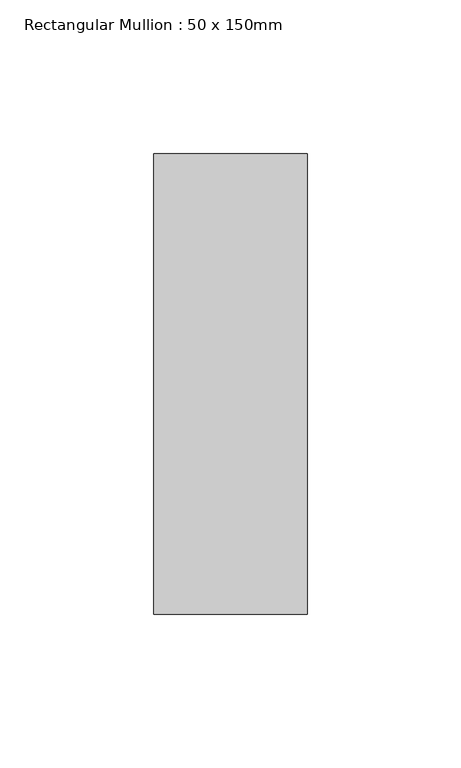
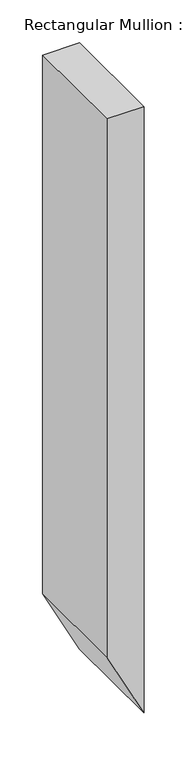
"""IFC4 building model written with IfcOpenShell, lengths in millimetres: member geometry, Rectangular Mullion : 50 x 150mm."""

from ifc_helpers import new_model, si_unit, frame, origin, place, context, project, spatial, polyline, outline, extrude, source, transform, mapped, element, save


def rectangular_mullion_50_x_150mm_a3343b62(model_context):
    return source(origin(), model_context, "Body", "SweptSolid", [
        extrude(outline(polyline([(0.0, 0.0), (0.0, -50.0), (-767.5359884, -50.0), (-863.5850948, 0.0), (0.0, 0.0)])), frame((0.0, -75.0, 0.0), z_axis=(0.0, 1.0, 0.0), x_axis=(0.0, 0.0, 1.0)), (0.0, 0.0, 1.0), 150.0),
    ])


if __name__ == "__main__":
    model = new_model("IFC4")
    model_context = context("Model", 3, world=origin())
    ifc_project = project(units=[si_unit("LENGTHUNIT", "METRE", prefix="MILLI")], contexts=[model_context])
    site = spatial("IfcSite", under=ifc_project)
    building = spatial("IfcBuilding", under=site)
    placement = place(None, origin())
    rectangular_mullion_50_x_150mm_shape = rectangular_mullion_50_x_150mm_a3343b62(model_context)
    element("IfcMember", 1, ObjectType="Rectangular Mullion : 50 x 150mm", at=placement, inside=building, context=model_context, shape_type="MappedRepresentation", body=[
        mapped(rectangular_mullion_50_x_150mm_shape, transform((0.0, 0.0, 0.0), x_axis=(1.0, 0.0, 0.0), y_axis=(0.0, 1.0, 0.0), z_axis=(0.0, 0.0, 1.0))),
    ])
    save(model, "model.ifc")

# Revit data of these elements
# Type "Rectangular Mullion : 50 x 150mm"
#   built-in parameter 1007304 = 0.492126 (stored number, unit not read)
#   built-in parameter 1007301 = 0.082021 (stored number, unit not read)
#   built-in parameter 1007300 = 0.082021 (stored number, unit not read)
# Element 1 (IfcMember, "Rectangular Mullion : 50 x 150mm")
#   Materials on its faces: "Aluminium"
# Materials
#   "Aluminium": class "Metal", colour RGB 247 247 247, transparency 0, Description = "Aluminium 6061", Cost = 0
